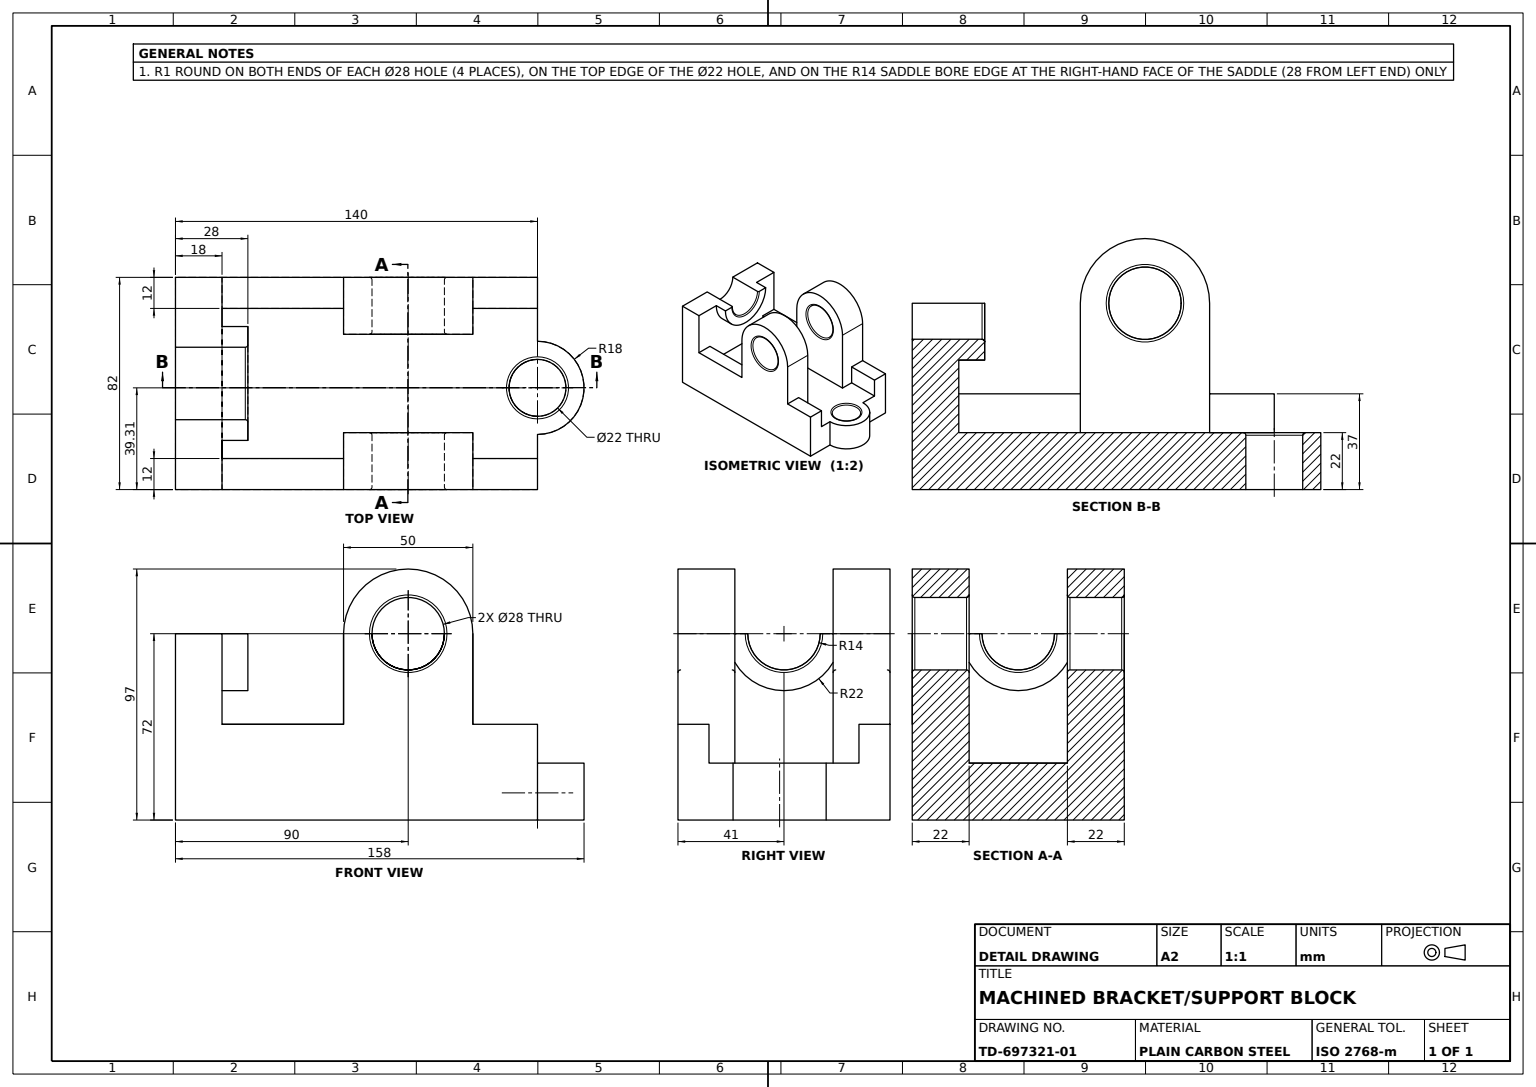
SolidWorks part; units mm, degrees
material "Plain Carbon Steel"
ref_plane "Front Plane" through (0, 0, 0) normal (0, 0, 1) x (1, 0, 0)
ref_plane "Top Plane" through (0, 0, 0) normal (0, 1, 0) x (1, 0, 0)
ref_plane "Right Plane" through (0, 0, 0) normal (1, 0, 0) x (0, 0, -1)
sketch "Base Block Sketch" plane through (0, 0, 0) normal (0, 1, 0) x (1, 0, 0)
  line L0 (70, 16.3082) -> (70, 41)
  line L2 (-70, -41) -> (70, -41)
  line L3 (-70, -41) -> (-70, 41)
  line L4 (-70, 41) -> (70, 41)
  line L5 (70, -41) -> (70, -19.6918)
  line L6 (-70, -41) -> (70, 41) construction
  line L7 (-70, 41) -> (70, -41) construction
  arc A0 (70, -19.6918) -> (70, 16.3082) centre (70, -1.6918) ccw
  circle A1 centre (70, -1.6918) radius 11
  point P1 (0, 0)
  dimension "D3" = 36
  dimension "D4" = 22
  dimension "D1" = 140
  dimension "D2" = 82
  dimension "D5" = 39.3082
extrude "Base Block" add sketch "Base Block Sketch" along normal blind 22
sketch "Side Walls Sketch" plane through (0, 22, 0) normal (0, 1, 0) x (1, 0, 0)
  line L0 (70, 29) -> (45, 29)
  line L1 (70, 16.3082) -> (70, 41) construction
  line L12 (70, -41) -> (70, -19.6918) construction
  line L13 (70, -29) -> (70, -41)
  line L14 (70, -41) -> (-70, -41)
  line L15 (-70, -41) -> (-70, 41)
  line L16 (-70, 41) -> (70, 41)
  line L17 (70, 41) -> (70, 29)
  line L18 (70, -29) -> (45, -29)
  line L19 (45, -29) -> (45, -19)
  line L20 (-52, 41) -> (-52, -41)
  line L21 (45, 29) -> (45, 41)
  line L22 (-5, 29) -> (-52, 29)
  line L23 (45, -19) -> (-5, -19)
  line L24 (45, 29) -> (45, 19)
  line L25 (45, 19) -> (-5, 19)
  line L26 (-5, 19) -> (-5, 41)
  line L27 (-5, -19) -> (-5, -29)
  line L28 (-5, -29) -> (-52, -29)
  line L29 (45, -29) -> (45, -41)
  line L30 (-5, -29) -> (-5, -41)
  line M29 (70, 41) -> (-70, 41)
  line M31 (-70, -41) -> (70, -41)
  line M32 (70, -41) -> (70, -19.6918)
  line M34 (70, 16.3082) -> (70, 41)
  dimension "D1" = 12
  dimension "D2" = 12
  dimension "D3" = 25
  dimension "D4" = 10
  dimension "D5" = 50
  dimension "D6" = 18
  dimension "D7" = 12
  dimension "D8" = 12
  dimension "D9" = 25
  dimension "D10" = 10
  dimension "D11" = 50
  dimension "D12" = 10
  dimension "D13" = 12
  dimension "D14" = 47
extrude "Side Walls" add sketch "Side Walls Sketch" along normal blind 15 contours L21 L0 M34 M29 | L22 L26 L20 M29 | L30 L28 L20 L14 | L18 L29 M31 M32
sketch "Uprights Sketch" plane through (0, 22, 0) normal (0, 1, 0) x (1, 0, 0)
  line L0 (-5, 41) -> (-5, 19)
  line L22 (-5, 19) -> (45, 19)
  line L23 (45, 19) -> (45, 41)
  line L24 (45, 41) -> (-5, 41)
  line L25 (-5, -19) -> (-5, -41)
  line L26 (-5, -41) -> (45, -41)
  line L27 (45, -41) -> (45, -19)
  line L28 (45, -19) -> (-5, -19)
  line L29 (-52, 41) -> (-52, -41)
  line L30 (-52, -29) -> (-52, -41) construction
  line L31 (-52, -41) -> (-70, -41)
  line L32 (-70, -41) -> (-70, 41)
  line L33 (-52, 41) -> (-70, 41) construction
  line L34 (-70, 41) -> (-70, -41) construction
  line L35 (-70, 41) -> (-52, 41)
  dimension "D1" = 22
  dimension "D2" = 22
  dimension "D3" = 22
  dimension "D4" = 18
extrude "Uprights" add sketch "Uprights Sketch" along normal blind 50
sketch "Pivot Lugs Sketch" plane through (0, 0, 41) normal (0, 0, 1) x (1, 0, 0)
  line L0 (-5, 72) -> (45, 72) construction
  line L1 (-5, 72) -> (6, 72)
  line L3 (34, 72) -> (45, 72)
  line L4 (-5, 72) -> (-5, 37)
  line L5 (-5, 37) -> (45, 37)
  line L6 (45, 72) -> (45, 37) construction
  line L7 (45, 37) -> (45, 72)
  line L8 (-5, 72) -> (-5, 37)
  line L9 (45, 72) -> (45, 37)
  arc A0 (45, 72) -> (-5, 72) centre (20, 72) ccw
  circle A1 centre (20, 72) radius 14
  dimension "D1" = 28
extrude "Pivot Lugs" add sketch "Pivot Lugs Sketch" against normal blind 22 contours A1 L4 A0
sketch "Lug Bore Sketch" plane through (0, 0, 41) normal (0, 0, 1) x (1, 0, 0)
  line L0 (6, 72) -> (34, 72) construction
  circle A0 centre (20, 72) radius 14
extrude "Lug Bore Through" cut sketch "Lug Bore Sketch" against normal blind 82
sketch "Lug Infill Sketch" plane through (0, 0, -41) normal (0, 0, -1) x (-1, 0, 0)
  line L0 (-34, 72) -> (-45, 72)
  line L1 (-6, 72) -> (5, 72)
  arc A0 (5, 72) -> (-45, 72) centre (-20, 72) ccw
  arc A1 (-6, 72) -> (-34, 72) centre (-20, 72) ccw
extrude "Lug Infill" add sketch "Lug Infill Sketch" against normal blind 22
sketch "Saddle Block Sketch" plane through (-70, 0, 0) normal (-1, 0, 0) x (0, 0, 1)
  line L0 (-41, 72) -> (41, 72) construction
  line L1 (-14, 72) -> (-22, 72)
  line L2 (14, 72) -> (22, 72)
  arc A0 (-22, 72) -> (22, 72) centre (0, 72) ccw
  arc A1 (-14, 72) -> (14, 72) centre (0, 72) ccw
  dimension "D1" = 44
  dimension "D2" = 28
extrude "Saddle Block" add sketch "Saddle Block Sketch" against normal blind 28
fillet "Base Edge Fillet R1" radius 1 1 edges at (70, 22, 12.6918)
fillet "Lug Edge Fillets R1" radius 1 5 edges at (-42, 58, 0) (6, 72, -19) (34, 72, 41) (34, 72, 19) (34, 72, -41)
sketch "Saddle Cradle Sketch" plane through (-52, 0, 0) normal (1, 0, 0) x (0, 0, -1)
  line L0 (-14, 72) -> (14, 72) construction
  line L1 (-14, 72) -> (14, 72)
  arc A0 (-14, 72) -> (14, 72) centre (0, 72) ccw
extrude "Saddle Cradle Cut" cut sketch "Saddle Cradle Sketch" against normal blind 22
